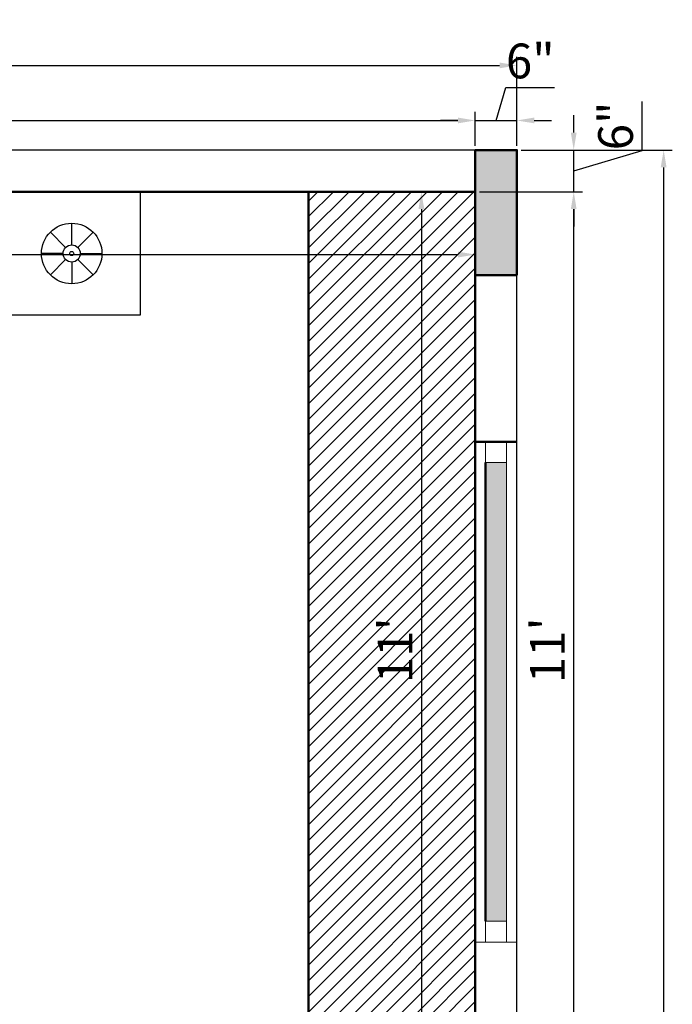
# Model space of a CAD drawing. Units: inches. Extents: x 3064 to 19385, y 846 to 15425.
# Tile 91 of 108: x 7370 to 7464, y 1273 to 1415. Entities that reach past the tile are written whole.
import ezdxf

# ---------------------------------------------------------------- set-up
doc = ezdxf.new("R2010")
doc.units = ezdxf.units.IN
for name, color, linetype, lineweight in [('A-ANNO-DIMS', 2, 'Continuous', 18), ('A-COLS', 1, 'Continuous', 35), ('A-FLOR-FIXT', 9, 'Continuous', 18), ('A-FURN-PATT', 252, 'Continuous', 13), ('A-GLAZ', 4, 'Continuous', 18), ('A-WALL', 7, 'Continuous', 50), ('C-PROP', 6, 'Continuous', 25)]:
    doc.layers.add(name, color=color, linetype=linetype, lineweight=lineweight)
doc.layers.add('BLOCK', color=6, linetype='Continuous')
doc.styles.get("Standard").update_dxf_attribs({"font": 'arial.ttf'})
doc.dimstyles.new('ISO-25', dxfattribs={"dimtxt": 9, "dimasz": 2.5, "dimexe": 1.25, "dimexo": 0.625, "dimtad": 1, "dimdec": 1, "dimlunit": 3, "dimtxsty": 'Standard', "dimcen": 2.5, "dimadec": 0, "dimazin": 0, "dimtfac": 1, "dimtdec": 1, "dimtmove": 0, "dimatfit": 3, "dimfxl": 1, "dimarcsym": 0})

# ---------------------------------------------------------------- blocks, each defined once
blk = doc.blocks.new('*D294')
at = {"layer": 'A-ANNO-DIMS', "color": 0, "lineweight": -2, "transparency": 16777216}
for p, q in [((7240.71, 1396.96), (7240.71, 1401.84)), ((7435.71, 1396.96), (7435.71, 1401.84)), ((7243.21, 1400.59), (7433.21, 1400.59))]:
    blk.add_line(p, q, dxfattribs=at)
at = {"layer": 'A-ANNO-DIMS', "color": 0, "transparency": 16777216}
for points in [[(7243.21, 1401.01), (7243.21, 1400.18), (7240.71, 1400.59)], [(7433.21, 1401.01), (7433.21, 1400.18), (7435.71, 1400.59)]]:
    blk.add_solid(points, dxfattribs=at)
at = {"layer": 'Defpoints', "color": 0, "transparency": 16777216}
for p in [(7435.71, 1400.59), (7240.71, 1396.34), (7435.71, 1396.34)]:
    blk.add_point(p, dxfattribs=at)
at = {"layer": 'A-ANNO-DIMS', "color": 0, "transparency": 16777216, "insert": (7338.21, 1403.77), "char_height": 5, "attachment_point": 5}
blk.add_mtext('16\'-3"', dxfattribs=at)
blk = doc.blocks.new('*D295')
at = {"layer": 'A-ANNO-DIMS', "color": 0, "lineweight": -2, "transparency": 16777216}
for p, q in [((7438.71, 1400.59), (7440.13, 1405.33)), ((7440.13, 1405.33), (7447.15, 1405.33)), ((7435.71, 1396.96), (7435.71, 1401.84)), ((7441.71, 1396.96), (7441.71, 1401.84)), ((7433.21, 1400.59), (7430.71, 1400.59)), ((7435.71, 1400.59), (7441.71, 1400.59)), ((7435.71, 1400.59), (7441.71, 1400.59)), ((7444.21, 1400.59), (7446.71, 1400.59))]:
    blk.add_line(p, q, dxfattribs=at)
at = {"layer": 'A-ANNO-DIMS', "color": 0, "transparency": 16777216}
for points in [[(7433.21, 1401.01), (7433.21, 1400.18), (7435.71, 1400.59)], [(7444.21, 1401.01), (7444.21, 1400.18), (7441.71, 1400.59)]]:
    blk.add_solid(points, dxfattribs=at)
at = {"layer": 'Defpoints', "color": 0, "transparency": 16777216}
for p in [(7441.71, 1400.59), (7435.71, 1396.34), (7441.71, 1396.34)]:
    blk.add_point(p, dxfattribs=at)
at = {"layer": 'A-ANNO-DIMS', "color": 0, "transparency": 16777216, "insert": (7443.64, 1408.51), "char_height": 5, "attachment_point": 5}
blk.add_mtext('6"', dxfattribs=at)
blk = doc.blocks.new('*D312')
at = {"layer": 'A-ANNO-DIMS', "color": 0, "lineweight": -2, "transparency": 16777216}
for p, q in [((7436.33, 1390.34), (7451.15, 1390.34)), ((7449.9, 1260.84), (7449.9, 1387.84)), ((7442.33, 1258.34), (7451.15, 1258.34))]:
    blk.add_line(p, q, dxfattribs=at)
at = {"layer": 'A-ANNO-DIMS', "color": 0, "transparency": 16777216}
for points in [[(7449.48, 1387.84), (7450.31, 1387.84), (7449.9, 1390.34)], [(7449.48, 1260.84), (7450.31, 1260.84), (7449.9, 1258.34)]]:
    blk.add_solid(points, dxfattribs=at)
at = {"layer": 'Defpoints', "color": 0, "transparency": 16777216}
for p in [(7435.71, 1390.34), (7449.9, 1390.34), (7441.71, 1258.34)]:
    blk.add_point(p, dxfattribs=at)
at = {"layer": 'A-ANNO-DIMS', "color": 0, "transparency": 16777216, "insert": (7446.76, 1324.34), "char_height": 5, "attachment_point": 5, "rotation": 90}
blk.add_mtext("11'", dxfattribs=at)
blk = doc.blocks.new('*D313')
at = {"layer": 'A-ANNO-DIMS', "color": 0, "lineweight": -2, "transparency": 16777216}
for p, q in [((7459.74, 1396.29), (7459.74, 1403.32)), ((7449.9, 1398.84), (7449.9, 1401.34)), ((7442.33, 1396.34), (7451.15, 1396.34)), ((7449.9, 1390.34), (7449.9, 1396.34)), ((7449.9, 1390.34), (7449.9, 1396.34)), ((7449.9, 1393.34), (7459.74, 1396.29)), ((7436.33, 1390.34), (7451.15, 1390.34)), ((7449.9, 1387.84), (7449.9, 1385.34))]:
    blk.add_line(p, q, dxfattribs=at)
at = {"layer": 'A-ANNO-DIMS', "color": 0, "transparency": 16777216}
for points in [[(7449.48, 1398.84), (7450.31, 1398.84), (7449.9, 1396.34)], [(7449.48, 1387.84), (7450.31, 1387.84), (7449.9, 1390.34)]]:
    blk.add_solid(points, dxfattribs=at)
at = {"layer": 'Defpoints', "color": 0, "transparency": 16777216}
for p in [(7441.71, 1396.34), (7449.9, 1396.34), (7435.71, 1390.34)]:
    blk.add_point(p, dxfattribs=at)
at = {"layer": 'A-ANNO-DIMS', "color": 0, "transparency": 16777216, "insert": (7456.57, 1399.81), "char_height": 5, "attachment_point": 5, "rotation": 90}
blk.add_mtext('6"', dxfattribs=at)
blk = doc.blocks.new('*D314')
at = {"layer": 'A-ANNO-DIMS', "color": 0, "lineweight": -2, "transparency": 16777216}
for p, q in [((7442.33, 1396.34), (7464.1, 1396.34)), ((7462.85, 1393.84), (7462.85, 882.84)), ((7442.33, 880.34), (7464.1, 880.34))]:
    blk.add_line(p, q, dxfattribs=at)
at = {"layer": 'A-ANNO-DIMS', "color": 0, "transparency": 16777216}
for points in [[(7462.43, 1393.84), (7463.27, 1393.84), (7462.85, 1396.34)], [(7462.43, 882.84), (7463.27, 882.84), (7462.85, 880.34)]]:
    blk.add_solid(points, dxfattribs=at)
at = {"layer": 'Defpoints', "color": 0, "transparency": 16777216}
for p in [(7441.71, 1396.34), (7441.71, 880.34), (7462.85, 880.34)]:
    blk.add_point(p, dxfattribs=at)
at = {"layer": 'A-ANNO-DIMS', "color": 0, "transparency": 16777216, "insert": (7459.67, 1138.34), "char_height": 5, "attachment_point": 5, "rotation": 90}
blk.add_mtext("43'", dxfattribs=at)
blk = doc.blocks.new('*D315')
at = {"layer": 'A-ANNO-DIMS', "color": 0, "lineweight": -2, "transparency": 16777216}
for p, q in [((7099.71, 1396.96), (7099.71, 1409.76)), ((7441.71, 1396.96), (7441.71, 1409.76)), ((7102.21, 1408.51), (7439.21, 1408.51))]:
    blk.add_line(p, q, dxfattribs=at)
at = {"layer": 'A-ANNO-DIMS', "color": 0, "transparency": 16777216}
for points in [[(7102.21, 1408.93), (7102.21, 1408.1), (7099.71, 1408.51)], [(7439.21, 1408.93), (7439.21, 1408.1), (7441.71, 1408.51)]]:
    blk.add_solid(points, dxfattribs=at)
at = {"layer": 'Defpoints', "color": 0, "transparency": 16777216}
for p in [(7441.71, 1408.51), (7099.71, 1396.34), (7441.71, 1396.34)]:
    blk.add_point(p, dxfattribs=at)
at = {"layer": 'A-ANNO-DIMS', "color": 0, "transparency": 16777216, "insert": (7270.71, 1411.69), "char_height": 5, "attachment_point": 5}
blk.add_mtext('28\'-6"', dxfattribs=at)
blk = doc.blocks.new('*D290')
at = {"layer": 'A-ANNO-DIMS', "color": 0, "lineweight": -2, "transparency": 16777216}
for p, q in [((7240.71, 1389.71), (7240.71, 1380.04)), ((7435.71, 1389.71), (7435.71, 1380.04)), ((7243.21, 1381.29), (7433.21, 1381.29))]:
    blk.add_line(p, q, dxfattribs=at)
at = {"layer": 'A-ANNO-DIMS', "color": 0, "transparency": 16777216}
for points in [[(7243.21, 1381.71), (7243.21, 1380.87), (7240.71, 1381.29)], [(7433.21, 1381.71), (7433.21, 1380.87), (7435.71, 1381.29)]]:
    blk.add_solid(points, dxfattribs=at)
at = {"layer": 'Defpoints', "color": 0, "transparency": 16777216}
for p in [(7240.71, 1390.34), (7435.71, 1390.34), (7435.71, 1381.29)]:
    blk.add_point(p, dxfattribs=at)
at = {"layer": 'A-ANNO-DIMS', "color": 0, "transparency": 16777216, "insert": (7338.21, 1384.47), "char_height": 5, "attachment_point": 5}
blk.add_mtext('16\'-3"', dxfattribs=at)
blk = doc.blocks.new('*D278')
at = {"layer": 'A-ANNO-DIMS', "color": 0, "lineweight": -2, "transparency": 16777216}
for p, q in [((7435.08, 1390.34), (7426.7, 1390.34)), ((7427.95, 1387.84), (7427.95, 1260.84)), ((7435.08, 1258.34), (7426.7, 1258.34))]:
    blk.add_line(p, q, dxfattribs=at)
at = {"layer": 'A-ANNO-DIMS', "color": 0, "transparency": 16777216}
for points in [[(7427.54, 1387.84), (7428.37, 1387.84), (7427.95, 1390.34)], [(7427.54, 1260.84), (7428.37, 1260.84), (7427.95, 1258.34)]]:
    blk.add_solid(points, dxfattribs=at)
at = {"layer": 'Defpoints', "color": 0, "transparency": 16777216}
for p in [(7435.71, 1390.34), (7427.95, 1258.34), (7435.71, 1258.34)]:
    blk.add_point(p, dxfattribs=at)
at = {"layer": 'A-ANNO-DIMS', "color": 0, "transparency": 16777216, "insert": (7424.82, 1324.34), "char_height": 5, "attachment_point": 5, "rotation": 90}
blk.add_mtext("11'", dxfattribs=at)
blk = doc.blocks.new('A$C52E67D0D')
at = {"layer": 'BLOCK'}
for p, q in [((2251.5, 1605.5), (2251.5, 1684.7)), ((2229.3, 1596.3), (2173.3, 1652.3)), ((2273.7, 1596.3), (2329.7, 1652.3)), ((2220.1, 1574.1), (2140.9, 1574.1)), ((2229.3, 1551.9), (2173.3, 1495.9)), ((2273.7, 1551.9), (2329.7, 1495.9)), ((2282.9, 1574.1), (2362.1, 1574.1)), ((2251.5, 1542.8), (2251.5, 1463.5))]:
    blk.add_line(p, q, dxfattribs=at)
blk.add_lwpolyline([(2001, 1348.6), (2001, 1799.6), (2502, 1799.6), (2502, 1348.6)], close=True, dxfattribs=at)
for radius in [110.6, 31.4, 7.46]:
    blk.add_circle((2251.5, 1574.1), radius, dxfattribs=at)
blk = doc.blocks.new('WIN-1900')
blk.add_line((3, 0), (3, 66))
blk.add_lwpolyline([(3, 66), (0, 66), (0, 69), (3, 69)], close=True)

msp = doc.modelspace()

# ---------------------------------------------------------------- hatches: boundary and pattern name
at = {"layer": 'A-COLS'}
h = msp.add_hatch(color=256, dxfattribs=at)
h.dxf.hatch_style = 1
h.paths.add_polyline_path([(7435.71, 1378.34), (7441.71, 1378.34), (7441.71, 1396.34), (7435.71, 1396.34)])
at = {"layer": 'A-FURN-PATT'}
h = msp.add_hatch(dxfattribs=at)
h.set_pattern_fill('ANSI31', color=256, scale=0.5)
h.set_pattern_definition([(45, (1784.0376, -1e-11), (-1.122532, 1.122532), [])])
h.paths.add_polyline_path([(7411.71, 1258.34), (7435.71, 1258.34), (7435.71, 1390.34), (7411.71, 1390.34)])
at = {"layer": 'A-GLAZ'}
h = msp.add_hatch(color=256, dxfattribs=at)
h.dxf.hatch_style = 1
h.paths.add_polyline_path([(7437.21, 1285.34), (7440.21, 1285.34), (7440.21, 1351.34), (7437.21, 1351.34)])

# ---------------------------------------------------------------- linework, layer by layer
msp.add_line((7441.71, 1282.34), (7435.71, 1282.34), dxfattribs=at)
msp.add_lwpolyline([(7440.21, 1282.34), (7437.21, 1282.34), (7437.21, 1285.34), (7440.21, 1285.34)], close=True, dxfattribs=at)
at = {"layer": 'A-WALL'}
for p, q in [((7435.71, 1390.34), (7240.71, 1390.34)), ((7411.71, 1252.34), (7411.71, 1390.34)), ((7435.71, 1258.34), (7435.71, 1390.34)), ((7435.71, 1354.34), (7441.71, 1354.34)), ((7437.21, 1351.34), (7437.21, 1285.34))]:
    msp.add_line(p, q, dxfattribs=at)
msp.add_lwpolyline([(7441.71, 1378.34), (7441.71, 1396.34), (7435.71, 1396.34), (7435.71, 1378.34)], close=True, dxfattribs=at)
at = {"layer": 'C-PROP'}
for p, q in [((7441.71, 1396.34), (7099.71, 1396.34)), ((7441.71, 880.34), (7441.71, 1396.34))]:
    msp.add_line(p, q, dxfattribs=at)

# ---------------------------------------------------------------- block references
at = {"layer": 'A-FLOR-FIXT', "xscale": 0.039370099999992, "yscale": 0.039370099999992, "zscale": 0.039370099999992}
msp.add_blockref('A$C52E67D0D', (7288.95, 1319.47), dxfattribs=at)
at = {"layer": 'A-GLAZ'}
msp.add_blockref('WIN-1900', (7437.2, 1285.34), dxfattribs=at)

# ---------------------------------------------------------------- dimensions: what is measured, and where the dimension line sits
at = {"layer": 'A-ANNO-DIMS'}
for base, p1, p2, override, picture, middle in [((7441.71, 1408.51), (7099.71, 1396.34), (7441.71, 1396.34), {"dimtxt": 5, "dimclrd": 0, "dimclre": 0, "dimclrt": 0}, '*D315', (7270.71, 1411.69)), ((7441.71, 1400.59), (7435.71, 1396.34), (7441.71, 1396.34), {"dimtxt": 5, "dimclrd": 0, "dimclre": 0, "dimclrt": 0, "dimtmove": 1}, '*D295', (7440.75, 1408.51)), ((7435.71, 1400.59), (7240.71, 1396.34), (7435.71, 1396.34), {"dimtxt": 5, "dimclrd": 0, "dimclre": 0, "dimclrt": 0, "dimtmove": 1}, '*D294', (7338.21, 1403.77)), ((7435.71, 1381.29), (7240.71, 1390.34), (7435.71, 1390.34), {"dimtxt": 5, "dimclrd": 0, "dimclre": 0, "dimclrt": 0}, '*D290', (7338.21, 1384.47))]:
    dim = msp.add_linear_dim(base=base, p1=p1, p2=p2, dimstyle='ISO-25', override=override, dxfattribs=at)
    dim.commit()
    dim.dimension.update_dxf_attribs({"geometry": picture, "text_midpoint": middle})
for base, p1, p2, override, picture, middle in [((7449.9, 1396.34), (7435.71, 1390.34), (7441.71, 1396.34), {"dimtxt": 5, "dimclrd": 0, "dimclre": 0, "dimclrt": 0, "dimtmove": 1}, '*D313', (7456.57, 1396.92)), ((7462.85, 880.34), (7441.71, 1396.34), (7441.71, 880.34), {"dimtxt": 5, "dimclrd": 0, "dimclre": 0, "dimclrt": 0}, '*D314', (7459.67, 1138.34)), ((7427.95, 1258.34), (7435.71, 1390.34), (7435.71, 1258.34), {"dimtxt": 5, "dimclrd": 0, "dimclre": 0, "dimclrt": 0}, '*D278', (7424.82, 1324.34)), ((7449.9, 1390.34), (7441.71, 1258.34), (7435.71, 1390.34), {"dimtxt": 5, "dimclrd": 0, "dimclre": 0, "dimclrt": 0, "dimtmove": 1}, '*D312', (7446.76, 1324.34))]:
    dim = msp.add_linear_dim(base=base, p1=p1, p2=p2, angle=90, dimstyle='ISO-25', override=override, dxfattribs=at)
    dim.commit()
    dim.dimension.update_dxf_attribs({"geometry": picture, "text_midpoint": middle})

doc.saveas('drawing.dxf')
